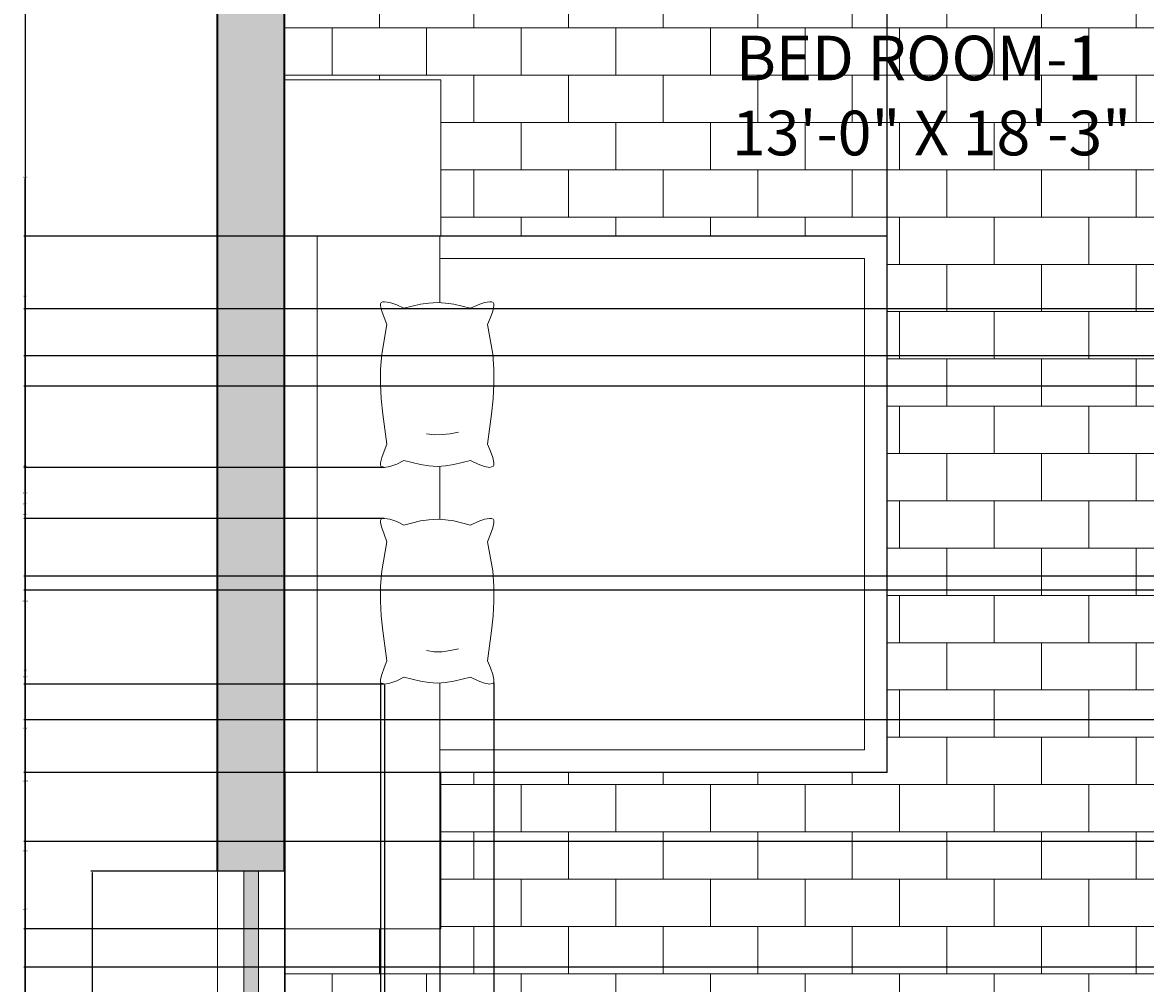
# Model space of a CAD drawing. Units: inches. Extents: x 6 to 575, y 34 to 566.
# Tile 3 of 21: x 6 to 157, y 258 to 387. Entities that reach past the tile are written whole.
import ezdxf

# ---------------------------------------------------------------- set-up
doc = ezdxf.new("R2010")
doc.units = ezdxf.units.IN
for name, color, linetype, lineweight in [('A-ANNO-DIMS', 2, 'Continuous', 18), ('A-AREA-IDEN', 6, 'Continuous', 20), ('A-FLOR-PATT', 252, 'Continuous', 9), ('A-GLAZ-PATT', 4, 'Continuous', 9), ('A-WALL-PATT', 251, 'Continuous', 9), ('FUR', 2, 'Continuous', 18), ('WALLS', 7, 'Continuous', 35), ('WINDOWS', 4, 'Continuous', 20)]:
    doc.layers.add(name, color=color, linetype=linetype, lineweight=lineweight)
doc.styles.add('PDF Arial Narrow', font='txt')
doc.styles.get("Standard").update_dxf_attribs({"font": 'arial.ttf'})
doc.dimstyles.get("Standard").update_dxf_attribs({"dimtxt": 0.18, "dimasz": 0.18, "dimexe": 0.18, "dimexo": 0.0625, "dimgap": 0.09, "dimtad": 0, "dimtih": 1, "dimtoh": 1, "dimdec": 4, "dimzin": 0, "dimdsep": 46, "dimtxsty": 'Standard', "dimcen": 0.09, "dimadec": 0, "dimazin": 0, "dimtfac": 1, "dimtdec": 4, "dimtofl": 0, "dimtmove": 0, "dimatfit": 3, "dimfxl": 1, "dimtolj": 1, "dimtzin": 0, "dimarcsym": 0})

# ---------------------------------------------------------------- blocks, each defined once
blk = doc.blocks.new('*D30')
at = {"layer": 'A-ANNO-DIMS', "color": 0, "lineweight": -2, "transparency": 16777216}
for p, q in [((32.6, 539.8), (6.65, 539.8)), ((6.83, 539.62), (6.83, 299.97)), ((6.83, 59.95), (6.83, 299.61)), ((197.62, 59.77), (6.65, 59.77))]:
    blk.add_line(p, q, dxfattribs=at)
at = {"layer": 'A-ANNO-DIMS', "color": 0, "transparency": 16777216}
for points in [[(6.8, 539.62), (6.86, 539.62), (6.83, 539.8)], [(6.8, 59.95), (6.86, 59.95), (6.83, 59.77)]]:
    blk.add_solid(points, dxfattribs=at)
at = {"layer": 'Defpoints', "color": 0, "transparency": 16777216}
for p in [(32.66, 539.8), (6.83, 59.77), (197.69, 59.77)]:
    blk.add_point(p, dxfattribs=at)
at = {"layer": 'A-ANNO-DIMS', "color": 0, "transparency": 16777216, "insert": (6.83, 299.79), "char_height": 0.18, "attachment_point": 5}
blk.add_mtext('\\A1;480', dxfattribs=at)
blk = doc.blocks.new('*D43')
at = {"layer": 'A-ANNO-DIMS', "color": 0, "lineweight": -2, "transparency": 16777216}
for p, q in [((41.6, 272.8), (15.65, 272.8)), ((15.83, 272.62), (15.83, 248.98)), ((15.83, 224.98), (15.83, 248.62)), ((41.6, 224.8), (15.65, 224.8))]:
    blk.add_line(p, q, dxfattribs=at)
at = {"layer": 'A-ANNO-DIMS', "color": 0, "transparency": 16777216}
for points in [[(15.8, 272.62), (15.86, 272.62), (15.83, 272.8)], [(15.8, 224.98), (15.86, 224.98), (15.83, 224.8)]]:
    blk.add_solid(points, dxfattribs=at)
at = {"layer": 'Defpoints', "color": 0, "transparency": 16777216}
for p in [(15.83, 272.8), (41.66, 272.8), (41.66, 224.8)]:
    blk.add_point(p, dxfattribs=at)
at = {"layer": 'A-ANNO-DIMS', "color": 0, "transparency": 16777216, "insert": (15.83, 248.8), "char_height": 0.18, "attachment_point": 5}
blk.add_mtext('\\A1;48', dxfattribs=at)
blk = doc.blocks.new('*D54')
at = {"layer": 'A-ANNO-DIMS', "color": 0, "lineweight": -2, "transparency": 16777216}
for p, q in [((444.96, 337.94), (6.65, 337.94)), ((6.83, 337.76), (6.83, 299.11)), ((6.83, 260.1), (6.83, 298.75)), ((444.96, 259.92), (6.65, 259.92))]:
    blk.add_line(p, q, dxfattribs=at)
at = {"layer": 'A-ANNO-DIMS', "color": 0, "transparency": 16777216}
for points in [[(6.8, 337.76), (6.86, 337.76), (6.83, 337.94)], [(6.8, 260.1), (6.86, 260.1), (6.83, 259.92)]]:
    blk.add_solid(points, dxfattribs=at)
at = {"layer": 'Defpoints', "color": 0, "transparency": 16777216}
for p in [(6.83, 337.94), (445.02, 337.94), (445.02, 259.92)]:
    blk.add_point(p, dxfattribs=at)
at = {"layer": 'A-ANNO-DIMS', "color": 0, "transparency": 16777216, "insert": (6.83, 298.93), "char_height": 0.18, "attachment_point": 5}
blk.add_mtext('\\A1;78.02', dxfattribs=at)
blk = doc.blocks.new('*D55')
at = {"layer": 'A-ANNO-DIMS', "color": 0, "lineweight": -2, "transparency": 16777216}
for p, q in [((41.66, 286.13), (41.66, 565.81)), ((41.84, 565.63), (81.79, 565.63)), ((122.38, 565.63), (82.44, 565.63)), ((122.56, 286.13), (122.56, 565.81))]:
    blk.add_line(p, q, dxfattribs=at)
at = {"layer": 'A-ANNO-DIMS', "color": 0, "transparency": 16777216}
for points in [[(41.84, 565.66), (41.84, 565.6), (41.66, 565.63)], [(122.38, 565.66), (122.38, 565.6), (122.56, 565.63)]]:
    blk.add_solid(points, dxfattribs=at)
at = {"layer": 'Defpoints', "color": 0, "transparency": 16777216}
for p in [(122.56, 565.63), (41.66, 286.06), (122.56, 286.06)]:
    blk.add_point(p, dxfattribs=at)
at = {"layer": 'A-ANNO-DIMS', "color": 0, "transparency": 16777216, "insert": (82.11, 565.63), "char_height": 0.18, "attachment_point": 5}
blk.add_mtext('\\A1;80.9', dxfattribs=at)
blk = doc.blocks.new('*D56')
at = {"layer": 'A-ANNO-DIMS', "color": 0, "lineweight": -2, "transparency": 16777216}
for p, q in [((122.5, 358.08), (6.65, 358.08)), ((6.83, 357.9), (6.83, 322.25)), ((6.83, 286.24), (6.83, 321.89)), ((122.5, 286.06), (6.65, 286.06))]:
    blk.add_line(p, q, dxfattribs=at)
at = {"layer": 'A-ANNO-DIMS', "color": 0, "transparency": 16777216}
for points in [[(6.8, 357.9), (6.86, 357.9), (6.83, 358.08)], [(6.8, 286.24), (6.86, 286.24), (6.83, 286.06)]]:
    blk.add_solid(points, dxfattribs=at)
at = {"layer": 'Defpoints', "color": 0, "transparency": 16777216}
for p in [(6.83, 358.08), (122.56, 358.08), (122.56, 286.06)]:
    blk.add_point(p, dxfattribs=at)
at = {"layer": 'A-ANNO-DIMS', "color": 0, "transparency": 16777216, "insert": (6.83, 322.07), "char_height": 0.18, "attachment_point": 5}
blk.add_mtext('\\A1;72.01', dxfattribs=at)
blk = doc.blocks.new('*D90')
at = {"layer": 'A-ANNO-DIMS', "color": 0, "lineweight": -2, "transparency": 16777216}
for p, q in [((41.6, 286.06), (6.65, 286.06)), ((6.83, 285.88), (6.83, 249.61)), ((6.83, 212.98), (6.83, 249.25)), ((41.6, 212.8), (6.65, 212.8))]:
    blk.add_line(p, q, dxfattribs=at)
at = {"layer": 'A-ANNO-DIMS', "color": 0, "transparency": 16777216}
for points in [[(6.8, 285.88), (6.86, 285.88), (6.83, 286.06)], [(6.8, 212.98), (6.86, 212.98), (6.83, 212.8)]]:
    blk.add_solid(points, dxfattribs=at)
at = {"layer": 'Defpoints', "color": 0, "transparency": 16777216}
for p in [(6.83, 286.06), (41.66, 286.06), (41.66, 212.8)]:
    blk.add_point(p, dxfattribs=at)
at = {"layer": 'A-ANNO-DIMS', "color": 0, "transparency": 16777216, "insert": (6.83, 249.43), "char_height": 0.18, "attachment_point": 5}
blk.add_mtext('\\A1;73.26', dxfattribs=at)
blk = doc.blocks.new('*D91')
at = {"layer": 'A-ANNO-DIMS', "color": 0, "lineweight": -2, "transparency": 16777216}
for p, q in [((62.49, 286), (62.49, 33.76)), ((41.66, 265.01), (41.66, 33.76)), ((41.84, 33.94), (51.68, 33.94)), ((62.31, 33.94), (52.47, 33.94))]:
    blk.add_line(p, q, dxfattribs=at)
at = {"layer": 'A-ANNO-DIMS', "color": 0, "transparency": 16777216}
for points in [[(41.84, 33.97), (41.84, 33.91), (41.66, 33.94)], [(62.31, 33.97), (62.31, 33.91), (62.49, 33.94)]]:
    blk.add_solid(points, dxfattribs=at)
at = {"layer": 'Defpoints', "color": 0, "transparency": 16777216}
for p in [(62.49, 286.06), (41.66, 265.08), (62.49, 33.94)]:
    blk.add_point(p, dxfattribs=at)
at = {"layer": 'A-ANNO-DIMS', "color": 0, "transparency": 16777216, "insert": (52.07, 33.94), "char_height": 0.18, "attachment_point": 5}
blk.add_mtext('\\A1;20.83', dxfattribs=at)
blk = doc.blocks.new('*D92')
at = {"layer": 'A-ANNO-DIMS', "color": 0, "lineweight": -2, "transparency": 16777216}
for p, q in [((41.6, 286.06), (6.65, 286.06)), ((6.83, 285.88), (6.83, 275.75)), ((6.83, 265.26), (6.83, 275.39)), ((41.6, 265.08), (6.65, 265.08))]:
    blk.add_line(p, q, dxfattribs=at)
at = {"layer": 'A-ANNO-DIMS', "color": 0, "transparency": 16777216}
for points in [[(6.8, 285.88), (6.86, 285.88), (6.83, 286.06)], [(6.8, 265.26), (6.86, 265.26), (6.83, 265.08)]]:
    blk.add_solid(points, dxfattribs=at)
at = {"layer": 'Defpoints', "color": 0, "transparency": 16777216}
for p in [(6.83, 286.06), (41.66, 286.06), (41.66, 265.08)]:
    blk.add_point(p, dxfattribs=at)
at = {"layer": 'A-ANNO-DIMS', "color": 0, "transparency": 16777216, "insert": (6.83, 275.57), "char_height": 0.18, "attachment_point": 5}
blk.add_mtext('\\A1;20.987', dxfattribs=at)
blk = doc.blocks.new('*D93')
at = {"layer": 'A-ANNO-DIMS', "color": 0, "lineweight": -2, "transparency": 16777216}
for p, q in [((54.53, 298.17), (54.53, 33.76)), ((69.75, 298.17), (69.75, 33.76)), ((54.71, 33.94), (61.68, 33.94)), ((69.57, 33.94), (62.59, 33.94))]:
    blk.add_line(p, q, dxfattribs=at)
at = {"layer": 'A-ANNO-DIMS', "color": 0, "transparency": 16777216}
for points in [[(54.71, 33.97), (54.71, 33.91), (54.53, 33.94)], [(69.57, 33.97), (69.57, 33.91), (69.75, 33.94)]]:
    blk.add_solid(points, dxfattribs=at)
at = {"layer": 'Defpoints', "color": 0, "transparency": 16777216}
for p in [(54.53, 298.24), (69.75, 298.24), (69.75, 33.94)]:
    blk.add_point(p, dxfattribs=at)
at = {"layer": 'A-ANNO-DIMS', "color": 0, "transparency": 16777216, "insert": (62.14, 33.94), "char_height": 0.18, "attachment_point": 5}
blk.add_mtext('\\A1;15.214', dxfattribs=at)
blk = doc.blocks.new('*D94')
at = {"layer": 'A-ANNO-DIMS', "color": 0, "lineweight": -2, "transparency": 16777216}
for p, q in [((55.02, 320.16), (6.65, 320.16)), ((6.83, 319.98), (6.83, 309.22)), ((6.83, 298.1), (6.83, 308.86)), ((55.02, 297.92), (6.65, 297.92))]:
    blk.add_line(p, q, dxfattribs=at)
at = {"layer": 'A-ANNO-DIMS', "color": 0, "transparency": 16777216}
for points in [[(6.8, 319.98), (6.86, 319.98), (6.83, 320.16)], [(6.8, 298.1), (6.86, 298.1), (6.83, 297.92)]]:
    blk.add_solid(points, dxfattribs=at)
at = {"layer": 'Defpoints', "color": 0, "transparency": 16777216}
for p in [(6.83, 320.16), (55.08, 320.16), (55.08, 297.92)]:
    blk.add_point(p, dxfattribs=at)
at = {"layer": 'A-ANNO-DIMS', "color": 0, "transparency": 16777216, "insert": (6.83, 309.04), "char_height": 0.18, "attachment_point": 5}
blk.add_mtext('\\A1;22.236', dxfattribs=at)
blk = doc.blocks.new('*D95')
at = {"layer": 'A-ANNO-DIMS', "color": 0, "lineweight": -2, "transparency": 16777216}
for p, q in [((55.02, 327.02), (6.65, 327.02)), ((6.83, 326.84), (6.83, 323.77)), ((6.83, 320.34), (6.83, 323.41)), ((55.02, 320.16), (6.65, 320.16))]:
    blk.add_line(p, q, dxfattribs=at)
at = {"layer": 'A-ANNO-DIMS', "color": 0, "transparency": 16777216}
for points in [[(6.8, 326.84), (6.86, 326.84), (6.83, 327.02)], [(6.8, 320.34), (6.86, 320.34), (6.83, 320.16)]]:
    blk.add_solid(points, dxfattribs=at)
at = {"layer": 'Defpoints', "color": 0, "transparency": 16777216}
for p in [(6.83, 327.02), (55.08, 327.02), (55.08, 320.16)]:
    blk.add_point(p, dxfattribs=at)
at = {"layer": 'A-ANNO-DIMS', "color": 0, "transparency": 16777216, "insert": (6.83, 323.59), "char_height": 0.18, "attachment_point": 5}
blk.add_mtext('\\A1;6.866', dxfattribs=at)
blk = doc.blocks.new('*D96')
at = {"layer": 'A-ANNO-DIMS', "color": 0, "lineweight": -2, "transparency": 16777216}
for p, q in [((55.02, 297.92), (6.65, 297.92)), ((6.83, 297.74), (6.83, 292.18)), ((6.83, 286.24), (6.83, 291.81)), ((62.43, 286.06), (6.65, 286.06))]:
    blk.add_line(p, q, dxfattribs=at)
at = {"layer": 'A-ANNO-DIMS', "color": 0, "transparency": 16777216}
for points in [[(6.8, 297.74), (6.86, 297.74), (6.83, 297.92)], [(6.8, 286.24), (6.86, 286.24), (6.83, 286.06)]]:
    blk.add_solid(points, dxfattribs=at)
at = {"layer": 'Defpoints', "color": 0, "transparency": 16777216}
for p in [(6.83, 297.92), (55.08, 297.92), (62.49, 286.06)]:
    blk.add_point(p, dxfattribs=at)
at = {"layer": 'A-ANNO-DIMS', "color": 0, "transparency": 16777216, "insert": (6.83, 291.99), "char_height": 0.18, "attachment_point": 5}
blk.add_mtext('\\A1;11.86', dxfattribs=at)
blk = doc.blocks.new('*D97')
at = {"layer": 'A-ANNO-DIMS', "color": 0, "lineweight": -2, "transparency": 16777216}
for p, q in [((55.08, 297.86), (55.08, 33.76)), ((41.66, 286), (41.66, 33.76)), ((41.84, 33.94), (47.98, 33.94)), ((54.9, 33.94), (48.75, 33.94))]:
    blk.add_line(p, q, dxfattribs=at)
at = {"layer": 'A-ANNO-DIMS', "color": 0, "transparency": 16777216}
for points in [[(41.84, 33.97), (41.84, 33.91), (41.66, 33.94)], [(54.9, 33.97), (54.9, 33.91), (55.08, 33.94)]]:
    blk.add_solid(points, dxfattribs=at)
at = {"layer": 'Defpoints', "color": 0, "transparency": 16777216}
for p in [(55.08, 297.92), (41.66, 286.06), (55.08, 33.94)]:
    blk.add_point(p, dxfattribs=at)
at = {"layer": 'A-ANNO-DIMS', "color": 0, "transparency": 16777216, "insert": (48.37, 33.94), "char_height": 0.18, "attachment_point": 5}
blk.add_mtext('\\A1;13.42', dxfattribs=at)
blk = doc.blocks.new('*D104')
at = {"layer": 'A-ANNO-DIMS', "color": 0, "lineweight": -2, "transparency": 16777216}
for p, q in [((197.64, 348.32), (6.65, 348.32)), ((6.83, 348.14), (6.83, 320.93)), ((6.83, 293.34), (6.83, 320.56)), ((182.58, 293.16), (6.65, 293.16))]:
    blk.add_line(p, q, dxfattribs=at)
at = {"layer": 'A-ANNO-DIMS', "color": 0, "transparency": 16777216}
for points in [[(6.8, 348.14), (6.86, 348.14), (6.83, 348.32)], [(6.8, 293.34), (6.86, 293.34), (6.83, 293.16)]]:
    blk.add_solid(points, dxfattribs=at)
at = {"layer": 'Defpoints', "color": 0, "transparency": 16777216}
for p in [(6.83, 348.32), (197.7, 348.32), (182.64, 293.16)]:
    blk.add_point(p, dxfattribs=at)
at = {"layer": 'A-ANNO-DIMS', "color": 0, "transparency": 16777216, "insert": (6.83, 320.74), "char_height": 0.18, "attachment_point": 5}
blk.add_mtext('\\A1;55.16', dxfattribs=at)
blk = doc.blocks.new('*D106')
at = {"layer": 'A-ANNO-DIMS', "color": 0, "lineweight": -2, "transparency": 16777216}
for p, q in [((197.64, 293.16), (6.65, 293.16)), ((6.83, 292.98), (6.83, 285.16)), ((6.83, 276.98), (6.83, 284.8)), ((197.6, 276.8), (6.65, 276.8))]:
    blk.add_line(p, q, dxfattribs=at)
at = {"layer": 'A-ANNO-DIMS', "color": 0, "transparency": 16777216}
for points in [[(6.8, 292.98), (6.86, 292.98), (6.83, 293.16)], [(6.8, 276.98), (6.86, 276.98), (6.83, 276.8)]]:
    blk.add_solid(points, dxfattribs=at)
at = {"layer": 'Defpoints', "color": 0, "transparency": 16777216}
for p in [(6.83, 293.16), (197.7, 293.16), (197.66, 276.8)]:
    blk.add_point(p, dxfattribs=at)
at = {"layer": 'A-ANNO-DIMS', "color": 0, "transparency": 16777216, "insert": (6.83, 284.98), "char_height": 0.18, "attachment_point": 5}
blk.add_mtext('\\A1;16.363', dxfattribs=at)
blk = doc.blocks.new('*D108')
at = {"layer": 'A-ANNO-DIMS', "color": 0, "lineweight": -2, "transparency": 16777216}
for p, q in [((197.6, 276.8), (6.65, 276.8)), ((6.83, 276.62), (6.83, 253.98)), ((6.83, 230.98), (6.83, 253.62)), ((197.6, 230.8), (6.65, 230.8))]:
    blk.add_line(p, q, dxfattribs=at)
at = {"layer": 'A-ANNO-DIMS', "color": 0, "transparency": 16777216}
for points in [[(6.8, 276.62), (6.86, 276.62), (6.83, 276.8)], [(6.8, 230.98), (6.86, 230.98), (6.83, 230.8)]]:
    blk.add_solid(points, dxfattribs=at)
at = {"layer": 'Defpoints', "color": 0, "transparency": 16777216}
for p in [(6.83, 276.8), (197.66, 276.8), (197.66, 230.8)]:
    blk.add_point(p, dxfattribs=at)
at = {"layer": 'A-ANNO-DIMS', "color": 0, "transparency": 16777216, "insert": (6.83, 253.8), "char_height": 0.18, "attachment_point": 5}
blk.add_mtext('\\A1;46', dxfattribs=at)
blk = doc.blocks.new('*D132')
at = {"layer": 'A-ANNO-DIMS', "color": 0, "lineweight": -2, "transparency": 16777216}
for p, q in [((288.54, 390), (6.65, 390)), ((6.83, 389.82), (6.83, 366.19)), ((6.83, 342.19), (6.83, 365.82)), ((288.54, 342.01), (6.65, 342.01))]:
    blk.add_line(p, q, dxfattribs=at)
at = {"layer": 'A-ANNO-DIMS', "color": 0, "transparency": 16777216}
for points in [[(6.8, 389.82), (6.86, 389.82), (6.83, 390)], [(6.8, 342.19), (6.86, 342.19), (6.83, 342.01)]]:
    blk.add_solid(points, dxfattribs=at)
at = {"layer": 'Defpoints', "color": 0, "transparency": 16777216}
for p in [(6.83, 390), (288.6, 390), (288.6, 342.01)]:
    blk.add_point(p, dxfattribs=at)
at = {"layer": 'A-ANNO-DIMS', "color": 0, "transparency": 16777216, "insert": (6.83, 366), "char_height": 0.18, "attachment_point": 5}
blk.add_mtext('\\A1;47.98', dxfattribs=at)
blk = doc.blocks.new('*D133')
at = {"layer": 'A-ANNO-DIMS', "color": 0, "lineweight": -2, "transparency": 16777216}
for p, q in [((288.54, 342.01), (6.65, 342.01)), ((6.83, 341.83), (6.83, 327.42)), ((6.83, 312.63), (6.83, 327.05)), ((288.79, 312.45), (6.65, 312.45))]:
    blk.add_line(p, q, dxfattribs=at)
at = {"layer": 'A-ANNO-DIMS', "color": 0, "transparency": 16777216}
for points in [[(6.8, 341.83), (6.86, 341.83), (6.83, 342.01)], [(6.8, 312.63), (6.86, 312.63), (6.83, 312.45)]]:
    blk.add_solid(points, dxfattribs=at)
at = {"layer": 'Defpoints', "color": 0, "transparency": 16777216}
for p in [(288.6, 342.01), (6.83, 312.45), (288.86, 312.45)]:
    blk.add_point(p, dxfattribs=at)
at = {"layer": 'A-ANNO-DIMS', "color": 0, "transparency": 16777216, "insert": (6.83, 327.23), "char_height": 0.18, "attachment_point": 5}
blk.add_mtext('\\A1;29.56', dxfattribs=at)
blk = doc.blocks.new('*D136')
at = {"layer": 'A-ANNO-DIMS', "color": 0, "lineweight": -2, "transparency": 16777216}
for p, q in [((206.62, 389.45), (6.65, 389.45)), ((6.83, 389.27), (6.83, 350.19)), ((6.83, 310.75), (6.83, 349.83)), ((206.62, 310.57), (6.65, 310.57))]:
    blk.add_line(p, q, dxfattribs=at)
at = {"layer": 'A-ANNO-DIMS', "color": 0, "transparency": 16777216}
for points in [[(6.8, 389.27), (6.86, 389.27), (6.83, 389.45)], [(6.8, 310.75), (6.86, 310.75), (6.83, 310.57)]]:
    blk.add_solid(points, dxfattribs=at)
at = {"layer": 'Defpoints', "color": 0, "transparency": 16777216}
for p in [(6.83, 389.45), (206.68, 389.45), (206.68, 310.57)]:
    blk.add_point(p, dxfattribs=at)
at = {"layer": 'A-ANNO-DIMS', "color": 0, "transparency": 16777216, "insert": (6.83, 350.01), "char_height": 0.18, "attachment_point": 5}
blk.add_mtext('\\A1;78.88', dxfattribs=at)
blk = doc.blocks.new('*D137')
at = {"layer": 'A-ANNO-DIMS', "color": 0, "lineweight": -2, "transparency": 16777216}
for p, q in [((206.62, 310.57), (6.65, 310.57)), ((6.83, 310.39), (6.83, 267.87)), ((6.83, 224.98), (6.83, 267.5)), ((206.6, 224.8), (6.65, 224.8))]:
    blk.add_line(p, q, dxfattribs=at)
at = {"layer": 'A-ANNO-DIMS', "color": 0, "transparency": 16777216}
for points in [[(6.8, 310.39), (6.86, 310.39), (6.83, 310.57)], [(6.8, 224.98), (6.86, 224.98), (6.83, 224.8)]]:
    blk.add_solid(points, dxfattribs=at)
at = {"layer": 'Defpoints', "color": 0, "transparency": 16777216}
for p in [(6.83, 310.57), (206.68, 310.57), (206.66, 224.8)]:
    blk.add_point(p, dxfattribs=at)
at = {"layer": 'A-ANNO-DIMS', "color": 0, "transparency": 16777216, "insert": (6.83, 267.69), "char_height": 0.18, "attachment_point": 5}
blk.add_mtext('\\A1;85.77', dxfattribs=at)

msp = doc.modelspace()

# ---------------------------------------------------------------- hatches: boundary and pattern name
at = {"layer": 'A-FLOR-PATT'}
h = msp.add_hatch(dxfattribs=at)
h.set_pattern_fill('BRICK', color=256)
h.set_pattern_definition([(0, (-98.035, 170.1465), (0, 6.35), []), (90, (-98.035, 170.147), (-12.7, 8e-16), [6.35, -6.35]), (90, (-91.685, 170.147), (-12.7, 8e-16), [-6.35, 6.35])])
h.paths.add_polyline_path([(180.8711, 269.7588), (182.4439, 270.6668), (182.4628, 270.6341, -0.11619827), (201.8275, 275.5902), (201.8275, 276.801), (197.6586, 276.801), (197.6586, 293.1641), (182.6401, 293.1641), (182.6401, 348.324), (197.6586, 348.324), (197.6586, 407.7709), (112.8513, 407.7709), (112.8513, 431.801), (111.6586, 431.801), (111.6586, 440.801), (117.6586, 440.801), (117.6586, 446.801), (117.6586, 448.2751), (117.6586, 473.3269), (117.6586, 474.801), (117.6586, 515.5941), (100.2533, 515.5941, -1), (83.0548, 515.5941), (65.6494, 515.5941), (65.6494, 440.801), (82.8918, 440.801), (82.8918, 431.801), (82.8918, 407.7709), (41.6586, 407.7709), (41.6586, 379.0637), (62.6459, 379.0637), (62.6459, 358.0764), (122.565, 358.0764), (122.565, 286.0643), (62.6459, 286.0643), (62.6459, 265.077), (41.6586, 265.077), (41.6586, 224.801), (41.6586, 212.801), (71.6586, 212.801), (167.6586, 212.801), (197.6586, 212.801), (197.6586, 230.801), (201.8157, 230.801), (201.8157, 233.4817)])
h.paths.add_polyline_path([(133.3414, 245.1275), (133.3317, 245.1352), (133.3317, 245.104)], flags=16)
h.paths.add_polyline_path([(133.3317, 222.1662), (85.3496, 222.1662), (85.3496, 243.7443, -0.50090726), (87.1831, 246.1963), (107.4292, 246.1963), (111.2522, 246.1963), (131.4202, 246.1963, -0.41421356), (133.3317, 244.2848)], flags=16)
h.paths.add_polyline_path([(72.7105, 244.4018), (72.7105, 220.3718), (48.6804, 220.3718), (48.6804, 244.4018)], flags=16)
h.paths.add_polyline_path([(71.7466, 237.8955, -1), (59.8096, 237.8955, -1)], flags=0)
at = {"layer": 'A-GLAZ-PATT'}
h = msp.add_hatch(color=256, dxfattribs=at)
h.dxf.hatch_style = 1
h.paths.add_polyline_path([(36.1586, 224.801), (38.1586, 224.801), (38.1586, 272.801), (36.1586, 272.801)])
h.paths.add_polyline_path([(167.6586, 207.301), (167.6586, 209.301), (71.6586, 209.301), (71.6586, 207.301)])
h.paths.add_polyline_path([(264.6586, 219.301), (264.6586, 221.301), (246.6586, 221.301), (246.6586, 219.301)])
h.paths.add_polyline_path([(316.6586, 221.301), (316.6586, 219.301), (334.6586, 219.301), (334.6586, 221.301)])
h.paths.add_polyline_path([(515.6586, 207.301), (515.6586, 209.301), (407.6586, 209.301), (407.6586, 207.301)])
h.paths.add_polyline_path([(543.1586, 270.801), (545.1586, 270.801), (545.1586, 366.801), (543.1586, 366.801)])
h.paths.add_polyline_path([(407.9436, 536.301), (407.9436, 534.301), (455.9436, 534.301), (455.9436, 536.301)])
h.paths.add_polyline_path([(272.6586, 536.301), (272.6586, 534.301), (320.6586, 534.301), (320.6586, 536.301)])
at = {"layer": 'A-WALL-PATT'}
h = msp.add_hatch(color=256, dxfattribs=at)
h.dxf.hatch_style = 1
h.paths.add_polyline_path([(160.6586, 539.801), (32.6586, 539.801), (32.6586, 272.801), (41.6586, 272.801), (41.6586, 286.0643), (41.6586, 358.0764), (41.6586, 379.0637), (41.6586, 407.7709), (41.6194, 407.7709), (41.6194, 431.801), (82.8918, 431.801), (82.8918, 440.801), (65.6494, 440.801), (65.6494, 440.7732), (41.6194, 440.7732), (41.6194, 515.5941), (41.6586, 530.801), (117.6586, 530.801), (117.6586, 474.801), (120.6068, 474.801), (121.6586, 474.801), (121.6586, 530.801), (137.4275, 530.801), (137.4275, 530.8356), (141.2505, 530.8356), (160.6586, 530.801)])
h.paths.add_polyline_path([(71.6586, 212.801), (41.6586, 212.801), (41.6586, 224.801), (32.6586, 224.801), (32.6586, 203.801), (71.6586, 203.801)])
h.paths.add_polyline_path([(206.6586, 215.801), (246.6586, 215.801), (246.6586, 224.801), (206.6586, 224.801), (206.6586, 230.801), (201.8157, 230.801), (197.6586, 230.801), (197.6586, 212.801), (167.6586, 212.801), (167.6586, 203.801), (206.6586, 203.801)])
h.paths.add_polyline_path([(383.6586, 224.801), (334.6586, 224.801), (334.6586, 215.801), (374.6586, 215.801), (374.6586, 203.801), (384.0753, 203.801), (407.6586, 203.801), (407.6586, 212.801), (383.6586, 212.801)])
h.paths.add_polyline_path([(548.6586, 270.801), (539.6586, 270.801), (539.6586, 212.801), (515.6586, 212.801), (515.6586, 203.801), (548.6586, 203.801)])
h.paths.add_polyline_path([(548.6586, 412.801), (545.7108, 412.801), (539.6586, 412.801), (539.6586, 382.801), (433.708, 382.801), (433.708, 378.801), (539.6586, 378.801), (539.6586, 366.801), (548.6586, 366.801)])
h.paths.add_polyline_path([(548.6586, 539.801), (455.9436, 539.801), (455.9436, 530.801), (539.6586, 530.801), (539.6586, 440.801), (548.6586, 440.801)])
h.paths.add_polyline_path([(407.9436, 539.801), (362.6586, 539.801), (362.6586, 530.801), (374.6586, 530.801), (374.6586, 452.801), (354.6586, 452.801), (354.6586, 448.801), (374.6586, 448.801), (374.6586, 278.801), (383.6586, 278.801), (383.6586, 530.801), (407.9436, 530.801)])
h.paths.add_polyline_path([(338.6586, 539.801), (320.6586, 539.801), (320.6586, 530.801), (322.6586, 530.801), (322.6586, 448.801), (326.6586, 448.801), (326.6586, 530.801), (338.6586, 530.801)])
h.paths.add_polyline_path([(272.6586, 539.801), (184.6586, 539.801), (184.6586, 530.801), (197.6586, 530.801), (197.6586, 440.801), (176.6714, 440.801), (121.6586, 440.801), (121.6586, 446.801), (117.6586, 446.801), (117.6586, 440.801), (111.6586, 440.801), (111.6586, 431.801), (197.6586, 431.801), (197.6586, 407.7709), (197.6586, 276.801), (206.6586, 276.801), (206.6586, 530.801), (272.6586, 530.801)])

# ---------------------------------------------------------------- linework, layer by layer
at = {"layer": 'FUR'}
for points in [[(62.6459, 358.0764), (41.6586, 358.0764), (41.6586, 379.0637), (62.6459, 379.0637)], [(41.6586, 358.0764), (46.0277, 358.0764), (46.0277, 286.0643), (41.6586, 286.0643)], [(66.6249, 327.9609), (64.3624, 327.4147), (63.2701, 327.2587), (62.1778, 327.1807), (61.0075, 327.2587), (59.9152, 327.4147), (57.6527, 327.9609), (56.7164, 327.4927), (55.7802, 327.1807), (55.078, 327.0246), (54.844, 327.1026), (54.6099, 327.1807), (54.5319, 327.3367), (54.5319, 327.6488), (54.6879, 328.351), (55, 329.2092), (55.3901, 330.1454), (54.844, 334.2024), (54.6099, 336.2309), (54.5319, 338.2594), (54.5319, 340.2099), (54.6879, 342.2385), (55.3901, 346.2175), (55, 347.1537), (54.6879, 348.0119), (54.5319, 348.7141), (54.5319, 349.0262), (54.6099, 349.1822), (54.844, 349.2602), (55.078, 349.2602), (55.7802, 349.1822), (56.7164, 348.8701), (57.6527, 348.402), (59.9152, 348.9481), (61.0075, 349.1042), (62.1778, 349.1822), (63.2701, 349.1042), (64.3624, 348.9481), (66.6249, 348.402), (67.6392, 348.8701), (68.4974, 349.1822), (69.1996, 349.2602), (69.4336, 349.2602), (69.6677, 349.1822), (69.7457, 349.0262), (69.7457, 348.7141), (69.5897, 348.0119), (69.2776, 347.1537), (68.8875, 346.2175), (69.5897, 342.2385), (69.7457, 340.2099), (69.7457, 338.2594), (69.6677, 336.2309), (69.4336, 334.2024), (68.8875, 330.1454), (69.2776, 329.2092), (69.5897, 328.351), (69.7457, 327.6488), (69.7457, 327.3367), (69.6677, 327.1807), (69.4336, 327.1026), (69.1996, 327.0246), (68.4974, 327.1807), (67.6392, 327.4927)], [(68.8875, 317.0381), (69.5897, 313.1371), (69.7457, 311.1086), (69.7457, 309.0801), (69.6677, 307.1296), (69.4336, 305.1011), (68.8875, 301.0441), (69.2776, 300.1079), (69.5897, 299.2496), (69.7457, 298.5475), (69.7457, 298.2354), (69.6677, 298.0793), (69.4336, 298.0013), (69.1996, 297.9233), (68.4974, 298.0793), (67.6392, 298.3914), (66.6249, 298.8595), (64.3624, 298.3134), (63.2701, 298.1574), (62.1778, 298.0793), (61.0075, 298.1574), (59.9152, 298.3134), (57.6527, 298.8595), (56.7164, 298.3914), (55.7802, 298.0793), (55.078, 297.9233), (54.844, 298.0013), (54.6099, 298.0793), (54.5319, 298.2354), (54.5319, 298.5475), (54.6879, 299.2496), (55, 300.1079), (55.3901, 301.0441), (54.844, 305.1011), (54.6099, 307.1296), (54.5319, 309.0801), (54.5319, 311.1086), (54.6879, 313.1371), (55.3901, 317.0381), (55, 318.0524), (54.6879, 318.9106), (54.5319, 319.6128), (54.5319, 319.9248), (54.6099, 320.0809), (54.844, 320.1589), (55.078, 320.1589), (55.7802, 320.0809), (56.7164, 319.7688), (57.6527, 319.3007), (59.9152, 319.8468), (61.0075, 320.0029), (62.1778, 320.0809), (63.2701, 320.0029), (64.3624, 319.8468), (66.6249, 319.3007), (67.6392, 319.7688), (68.4974, 320.0809), (69.1996, 320.1589), (69.4336, 320.1589), (69.6677, 320.0809), (69.7457, 319.9248), (69.7457, 319.6128), (69.5897, 318.9106), (69.2776, 318.0524)], [(62.6459, 286.0643), (41.6586, 286.0643), (41.6586, 265.077), (62.6459, 265.077)]]:
    msp.add_lwpolyline(points, close=True, dxfattribs=at)
for points in [[(62.4899, 358.0764), (122.565, 358.0764), (122.565, 286.0643), (62.4899, 286.0643)], [(62.4899, 358.0764), (62.4899, 349.1822)], [(62.4899, 355.1117), (119.5222, 355.1117), (119.5222, 289.1071), (62.4899, 289.1071)], [(64.9865, 331.7838), (63.8942, 331.5498), (62.802, 331.4717), (61.7097, 331.3937), (60.6954, 331.5498)], [(62.4899, 327.1807), (62.4899, 320.0809)], [(64.9865, 302.6825), (63.8942, 302.4484), (62.802, 302.2924), (61.7097, 302.2924), (60.6954, 302.4484)], [(62.4899, 298.0793), (62.4899, 286.0643)]]:
    msp.add_lwpolyline(points, dxfattribs=at)
at = {"layer": 'WALLS'}
for p, q in [((32.6586, 272.801), (32.6586, 539.801)), ((41.6586, 272.801), (41.6586, 431.801))]:
    msp.add_line(p, q, dxfattribs=at)
at = {"layer": 'WINDOWS'}
for p, q in [((41.6586, 272.801), (32.6586, 272.801)), ((36.1586, 224.801), (36.1586, 272.801)), ((38.1586, 224.801), (38.1586, 272.801))]:
    msp.add_line(p, q, dxfattribs=at)
msp.add_lwpolyline([(32.6586, 224.801), (41.6586, 224.801), (41.6586, 272.801), (32.6586, 272.801)], close=True, dxfattribs=at)

# ---------------------------------------------------------------- texts
at = {"layer": 'A-AREA-IDEN', "attachment_point": 4, "style": 'PDF Arial Narrow'}
for s, insert, char_height in [('BED ROOM-1', (102.2495, 381.2306), 6.0005), ('13\'-0" X 18\'-3"', (101.7033, 371.1656), 6.000503)]:
    msp.add_mtext(s, dxfattribs=dict(at, insert=insert, char_height=char_height))

# ---------------------------------------------------------------- dimensions: what is measured, and where the dimension line sits
at = {"layer": 'A-ANNO-DIMS'}
for base, p1, p2, override, picture, middle in [((122.565, 565.631), (41.6586, 286.0643), (122.565, 286.0643), {"dimdec": 1, "dimlfac": 1, "dimrnd": 0, "dimzin": 0, "dimdsep": 46, "dimlunit": 2}, '*D55', (82.1118, 565.631)), ((55.078, 33.9447), (41.6586, 286.0643), (55.078, 297.9233), {"dimdec": 2, "dimlfac": 1, "dimrnd": 0, "dimzin": 0, "dimdsep": 46, "dimlunit": 2}, '*D97', (48.3683, 33.9447)), ((69.7457, 33.9447), (54.5319, 298.2354), (69.7457, 298.2354), {"dimdec": 3, "dimlfac": 1, "dimrnd": 0, "dimzin": 0, "dimdsep": 46, "dimlunit": 2}, '*D93', (62.1388, 33.9447)), ((62.4899, 33.9447), (41.6586, 265.077), (62.4899, 286.0643), {"dimdec": 2, "dimlfac": 1, "dimrnd": 0, "dimzin": 0, "dimdsep": 46, "dimlunit": 2}, '*D91', (52.0743, 33.9447))]:
    dim = msp.add_linear_dim(base=base, p1=p1, p2=p2, dimstyle='Standard', override=override, dxfattribs=at)
    dim.commit()
    dim.dimension.update_dxf_attribs({"geometry": picture, "text_midpoint": middle})
for base, p1, p2, override, picture, middle in [((6.8286, 59.7747), (32.6586, 539.801), (197.6872, 59.7747), {"dimdec": 0, "dimlfac": 1, "dimrnd": 0, "dimzin": 0, "dimdsep": 46, "dimlunit": 2}, '*D30', (6.8286, 299.7878)), ((6.8286, 389.9952), (288.603, 342.0131), (288.603, 389.9952), {"dimdec": 2, "dimlfac": 1, "dimrnd": 0, "dimzin": 0, "dimdsep": 46, "dimlunit": 2}, '*D132', (6.8286, 366.0042)), ((6.8286, 389.449), (206.6824, 310.5712), (206.6824, 389.449), {"dimdec": 2, "dimlfac": 1, "dimrnd": 0, "dimzin": 0, "dimdsep": 46, "dimlunit": 2}, '*D136', (6.8286, 350.0101)), ((6.8286, 358.0764), (122.565, 286.0643), (122.565, 358.0764), {"dimdec": 2, "dimlfac": 1, "dimrnd": 0, "dimzin": 0, "dimdsep": 46, "dimlunit": 2}, '*D56', (6.8286, 322.0704)), ((6.8286, 348.324), (182.6401, 293.1641), (197.6979, 348.324), {"dimdec": 2, "dimlfac": 1, "dimrnd": 0, "dimzin": 0, "dimdsep": 46, "dimlunit": 2}, '*D104', (6.8286, 320.744)), ((6.8286, 312.455), (288.603, 342.0131), (288.8575, 312.455), {"dimdec": 2, "dimlfac": 1, "dimrnd": 0, "dimzin": 0, "dimdsep": 46, "dimlunit": 2}, '*D133', (6.8286, 327.234)), ((6.8286, 337.9397), (445.0208, 259.9201), (445.0208, 337.9397), {"dimdec": 2, "dimlfac": 1, "dimrnd": 0, "dimzin": 0, "dimdsep": 46, "dimlunit": 2}, '*D54', (6.8286, 298.9299)), ((6.8286, 327.0246), (55.078, 320.1589), (55.078, 327.0246), {"dimdec": 3, "dimlfac": 1, "dimrnd": 0, "dimzin": 0, "dimdsep": 46, "dimlunit": 2}, '*D95', (6.8286, 323.5918)), ((6.8286, 320.1589), (55.078, 297.9233), (55.078, 320.1589), {"dimdec": 3, "dimlfac": 1, "dimrnd": 0, "dimzin": 0, "dimdsep": 46, "dimlunit": 2}, '*D94', (6.8286, 309.0411)), ((6.8286, 310.5712), (206.6586, 224.801), (206.6824, 310.5712), {"dimdec": 2, "dimlfac": 1, "dimrnd": 0, "dimzin": 0, "dimdsep": 46, "dimlunit": 2}, '*D137', (6.8286, 267.6861)), ((6.8286, 297.9233), (62.4899, 286.0643), (55.078, 297.9233), {"dimdec": 2, "dimlfac": 1, "dimrnd": 0, "dimzin": 0, "dimdsep": 46, "dimlunit": 2}, '*D96', (6.8286, 291.9938)), ((6.8286, 293.1641), (197.6586, 276.801), (197.6979, 293.1641), {"dimdec": 3, "dimlfac": 1, "dimrnd": 0, "dimzin": 0, "dimdsep": 46, "dimlunit": 2}, '*D106', (6.8286, 284.9825)), ((6.8286, 286.0643), (41.6586, 265.077), (41.6586, 286.0643), {"dimdec": 3, "dimlfac": 1, "dimrnd": 0, "dimzin": 0, "dimdsep": 46, "dimlunit": 2}, '*D92', (6.8286, 275.5707)), ((6.8286, 286.0643), (41.6586, 212.801), (41.6586, 286.0643), {"dimdec": 2, "dimlfac": 1, "dimrnd": 0, "dimzin": 0, "dimdsep": 46, "dimlunit": 2}, '*D90', (6.8286, 249.4327)), ((6.8286, 276.801), (197.6586, 230.801), (197.6586, 276.801), {"dimdec": 0, "dimlfac": 1, "dimrnd": 0, "dimzin": 0, "dimdsep": 46, "dimlunit": 2}, '*D108', (6.8286, 253.801)), ((15.8286, 272.801), (41.6586, 224.801), (41.6586, 272.801), {"dimdec": 0, "dimlfac": 1, "dimrnd": 0, "dimzin": 0, "dimdsep": 46, "dimlunit": 2}, '*D43', (15.8286, 248.801))]:
    dim = msp.add_linear_dim(base=base, p1=p1, p2=p2, angle=90, dimstyle='Standard', override=override, dxfattribs=at)
    dim.commit()
    dim.dimension.update_dxf_attribs({"geometry": picture, "text_midpoint": middle})

doc.saveas('drawing.dxf')
